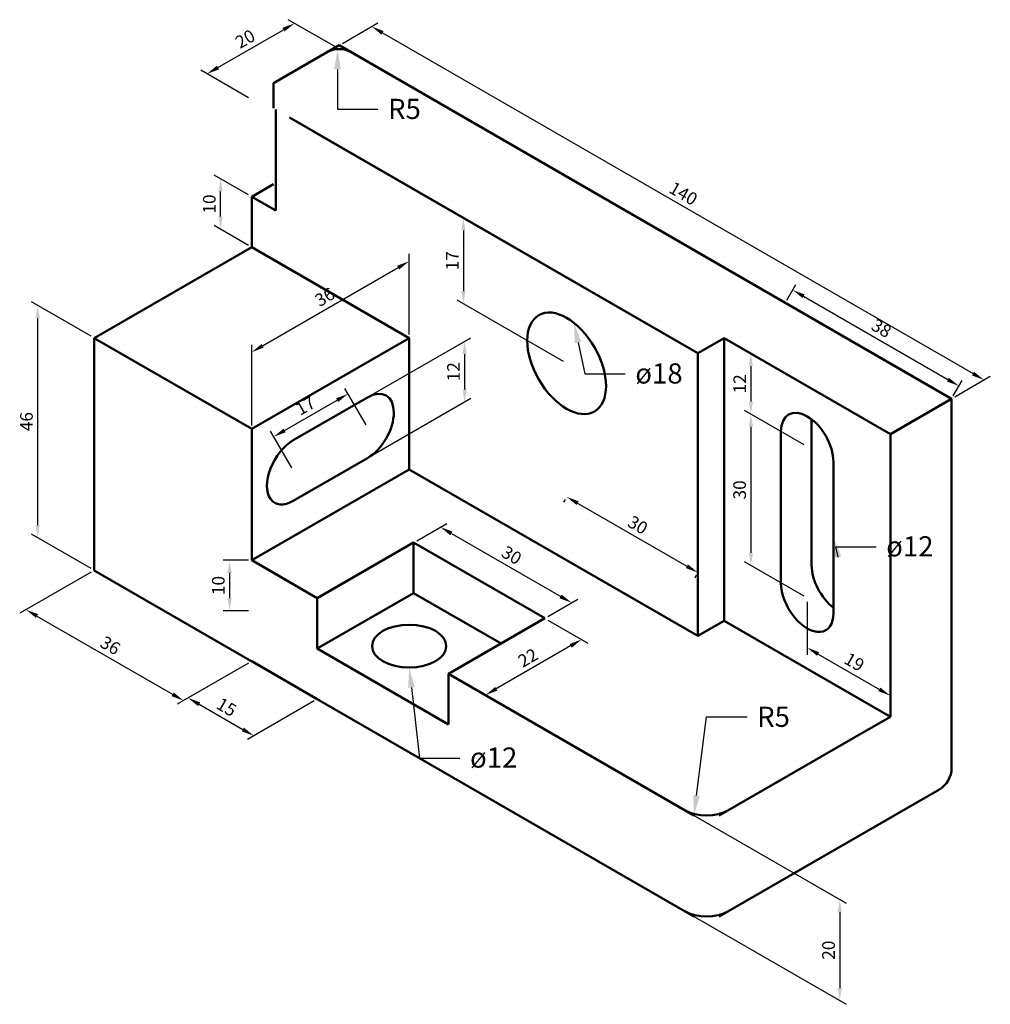
# Model space of a CAD drawing. Units: millimetres. Extents: x 2409 to 2602, y 2299 to 2494.
import ezdxf
from ezdxf import colors
from ezdxf.entities.mleader import LeaderData, LeaderLine
from ezdxf.math import Vec2, Vec3

# ---------------------------------------------------------------- set-up
doc = ezdxf.new("R2010")
doc.units = ezdxf.units.MM
for name, color, linetype, lineweight in [('M-DIMS', 2, 'Continuous', 25), ('M-OUTL', 7, 'Continuous', 50), ('M-TEXT', 3, 'Continuous', 25)]:
    doc.layers.add(name, color=color, linetype=linetype, lineweight=lineweight)
doc.styles.get("Standard").update_dxf_attribs({"font": 'arial.ttf'})
doc.dimstyles.new('ISO-25', dxfattribs={"dimtxt": 2.5, "dimasz": 2.5, "dimexe": 1.25, "dimexo": 0.625, "dimtad": 1, "dimtxsty": 'Standard', "dimcen": 2.5, "dimadec": 0, "dimazin": 0, "dimtfac": 1, "dimtmove": 0, "dimatfit": 3, "dimfxl": 1, "dimarcsym": 0})

# ---------------------------------------------------------------- blocks, each defined once
blk = doc.blocks.new('*D1')
at = {"layer": 'Defpoints', "color": 0, "transparency": 16777216}
for p in [(2486.5, 2446.55), (2486.5, 2431.33), (2455.32, 2413.33)]:
    blk.add_point(p, dxfattribs=at)
at = {"layer": 'M-DIMS', "color": 0, "lineweight": -2, "transparency": 16777216}
for p, q in [((2486.5, 2432.05), (2486.5, 2447.99)), ((2457.49, 2429.8), (2484.33, 2445.3)), ((2455.32, 2414.05), (2455.32, 2429.99))]:
    blk.add_line(p, q, dxfattribs=at)
at = {"layer": 'M-DIMS', "color": 0, "transparency": 16777216}
for points in [[(2484.12, 2445.66), (2484.54, 2444.94), (2486.5, 2446.55)], [(2457.28, 2430.16), (2457.69, 2429.44), (2455.32, 2428.55)]]:
    blk.add_solid(points, dxfattribs=at)
at = {"layer": 'M-DIMS', "color": 0, "transparency": 16777216, "insert": (2469.96, 2439.2), "char_height": 2.5, "attachment_point": 5, "rotation": 30}
blk.add_mtext('36', dxfattribs=at)
blk = doc.blocks.new('*D2')
at = {"layer": 'Defpoints', "color": 0, "transparency": 16777216}
for p in [(2412.96, 2437.79), (2424.14, 2431.33), (2424.14, 2385.33)]:
    blk.add_point(p, dxfattribs=at)
at = {"layer": 'M-DIMS', "color": 0, "lineweight": -2, "transparency": 16777216}
for p, q in [((2423.52, 2431.69), (2411.71, 2438.51)), ((2412.96, 2394.29), (2412.96, 2435.29)), ((2423.52, 2385.69), (2411.71, 2392.51))]:
    blk.add_line(p, q, dxfattribs=at)
at = {"layer": 'M-DIMS', "color": 0, "transparency": 16777216}
for points in [[(2412.54, 2435.29), (2413.37, 2435.29), (2412.96, 2437.79)], [(2412.54, 2394.29), (2413.37, 2394.29), (2412.96, 2391.79)]]:
    blk.add_solid(points, dxfattribs=at)
at = {"layer": 'M-DIMS', "color": 0, "transparency": 16777216, "insert": (2411.05, 2414.79), "char_height": 2.5, "attachment_point": 5, "rotation": 90}
blk.add_mtext('46', dxfattribs=at)
blk = doc.blocks.new('*D3')
at = {"layer": 'Defpoints', "color": 0, "transparency": 16777216}
for p in [(2424.14, 2385.33), (2455.32, 2367.33), (2441.82, 2359.54)]:
    blk.add_point(p, dxfattribs=at)
at = {"layer": 'M-DIMS', "color": 0, "lineweight": -2, "transparency": 16777216}
for p, q in [((2423.52, 2384.97), (2409.39, 2376.82)), ((2412.81, 2376.29), (2439.65, 2360.79)), ((2454.7, 2366.97), (2440.57, 2358.82))]:
    blk.add_line(p, q, dxfattribs=at)
at = {"layer": 'M-DIMS', "color": 0, "transparency": 16777216}
for points in [[(2413.02, 2376.65), (2412.6, 2375.93), (2410.64, 2377.54)], [(2439.86, 2361.15), (2439.45, 2360.43), (2441.82, 2359.54)]]:
    blk.add_solid(points, dxfattribs=at)
at = {"layer": 'M-DIMS', "color": 0, "transparency": 16777216, "insert": (2427.18, 2370.18), "char_height": 2.5, "attachment_point": 5, "rotation": 330}
blk.add_mtext('36', dxfattribs=at)
blk = doc.blocks.new('*D4')
at = {"layer": 'Defpoints', "color": 0, "transparency": 16777216}
for p in [(2455.32, 2367.33), (2468.31, 2359.83), (2455.73, 2352.57)]:
    blk.add_point(p, dxfattribs=at)
at = {"layer": 'M-DIMS', "color": 0, "lineweight": -2, "transparency": 16777216}
for p, q in [((2454.7, 2366.97), (2441.49, 2359.35)), ((2467.69, 2359.47), (2454.48, 2351.85)), ((2444.91, 2358.82), (2453.57, 2353.82))]:
    blk.add_line(p, q, dxfattribs=at)
at = {"layer": 'M-DIMS', "color": 0, "transparency": 16777216}
for points in [[(2445.12, 2359.18), (2444.7, 2358.46), (2442.74, 2360.07)], [(2453.78, 2354.18), (2453.36, 2353.46), (2455.73, 2352.57)]]:
    blk.add_solid(points, dxfattribs=at)
at = {"layer": 'M-DIMS', "color": 0, "transparency": 16777216, "insert": (2450.19, 2357.97), "char_height": 2.5, "attachment_point": 5, "rotation": 330}
blk.add_mtext('15', dxfattribs=at)
blk = doc.blocks.new('*D5')
at = {"layer": 'Defpoints', "color": 0, "transparency": 16777216}
for p in [(2455.32, 2387.33), (2450.95, 2377.33), (2455.32, 2377.33)]:
    blk.add_point(p, dxfattribs=at)
at = {"layer": 'M-DIMS', "color": 0, "lineweight": -2, "transparency": 16777216}
for p, q in [((2454.7, 2387.33), (2449.7, 2387.33)), ((2450.95, 2384.83), (2450.95, 2379.83)), ((2454.7, 2377.33), (2449.7, 2377.33))]:
    blk.add_line(p, q, dxfattribs=at)
at = {"layer": 'M-DIMS', "color": 0, "transparency": 16777216}
for points in [[(2450.53, 2384.83), (2451.36, 2384.83), (2450.95, 2387.33)], [(2450.53, 2379.83), (2451.36, 2379.83), (2450.95, 2377.33)]]:
    blk.add_solid(points, dxfattribs=at)
at = {"layer": 'M-DIMS', "color": 0, "transparency": 16777216, "insert": (2449.04, 2382.33), "char_height": 2.5, "attachment_point": 5, "rotation": 90}
blk.add_mtext('10', dxfattribs=at)
blk = doc.blocks.new('*D6')
at = {"layer": 'Defpoints', "color": 0, "transparency": 16777216}
for p in [(2487.36, 2390.83), (2518.67, 2378.91), (2513.34, 2375.83)]:
    blk.add_point(p, dxfattribs=at)
at = {"layer": 'M-DIMS', "color": 0, "lineweight": -2, "transparency": 16777216}
for p, q in [((2487.99, 2391.19), (2493.94, 2394.63)), ((2494.85, 2392.66), (2516.5, 2380.16)), ((2513.97, 2376.19), (2519.92, 2379.63))]:
    blk.add_line(p, q, dxfattribs=at)
at = {"layer": 'M-DIMS', "color": 0, "transparency": 16777216}
for points in [[(2495.06, 2393.02), (2494.64, 2392.29), (2492.69, 2393.91)], [(2516.71, 2380.52), (2516.29, 2379.79), (2518.67, 2378.91)]]:
    blk.add_solid(points, dxfattribs=at)
at = {"layer": 'M-DIMS', "color": 0, "transparency": 16777216, "insert": (2506.63, 2388.05), "char_height": 2.5, "attachment_point": 5, "rotation": 330}
blk.add_mtext('30', dxfattribs=at)
blk = doc.blocks.new('*D7')
at = {"layer": 'Defpoints', "color": 0, "transparency": 16777216}
for p in [(2513.34, 2375.83), (2494.29, 2364.83), (2501.58, 2360.62)]:
    blk.add_point(p, dxfattribs=at)
at = {"layer": 'M-DIMS', "color": 0, "lineweight": -2, "transparency": 16777216}
for p, q in [((2513.97, 2375.47), (2521.88, 2370.9)), ((2518.47, 2370.37), (2503.75, 2361.87)), ((2494.92, 2364.47), (2502.83, 2359.9))]:
    blk.add_line(p, q, dxfattribs=at)
at = {"layer": 'M-DIMS', "color": 0, "transparency": 16777216}
for points in [[(2518.26, 2370.74), (2518.68, 2370.01), (2520.63, 2371.62)], [(2503.54, 2362.24), (2503.95, 2361.51), (2501.58, 2360.62)]]:
    blk.add_solid(points, dxfattribs=at)
at = {"layer": 'M-DIMS', "color": 0, "transparency": 16777216, "insert": (2510.17, 2367.75), "char_height": 2.5, "attachment_point": 5, "rotation": 30}
blk.add_mtext('22', dxfattribs=at)
blk = doc.blocks.new('*D8')
at = {"layer": 'Defpoints', "color": 0, "transparency": 16777216}
for p in [(2449.16, 2462.89), (2455.32, 2459.33), (2455.32, 2449.33)]:
    blk.add_point(p, dxfattribs=at)
at = {"layer": 'M-DIMS', "color": 0, "lineweight": -2, "transparency": 16777216}
for p, q in [((2454.7, 2459.69), (2447.91, 2463.61)), ((2449.16, 2455.39), (2449.16, 2460.39)), ((2454.7, 2449.69), (2447.91, 2453.61))]:
    blk.add_line(p, q, dxfattribs=at)
at = {"layer": 'M-DIMS', "color": 0, "transparency": 16777216}
for points in [[(2448.75, 2460.39), (2449.58, 2460.39), (2449.16, 2462.89)], [(2448.75, 2455.39), (2449.58, 2455.39), (2449.16, 2452.89)]]:
    blk.add_solid(points, dxfattribs=at)
at = {"layer": 'M-DIMS', "color": 0, "transparency": 16777216, "insert": (2447.26, 2457.89), "char_height": 2.5, "attachment_point": 5, "rotation": 90}
blk.add_mtext('10', dxfattribs=at)
blk = doc.blocks.new('*D9')
at = {"layer": 'Defpoints', "color": 0, "transparency": 16777216}
for p in [(2463.8, 2493.66), (2472.64, 2488.56), (2455.32, 2478.56)]:
    blk.add_point(p, dxfattribs=at)
at = {"layer": 'M-DIMS', "color": 0, "lineweight": -2, "transparency": 16777216}
for p, q in [((2472.02, 2488.92), (2462.55, 2494.39)), ((2448.64, 2484.91), (2461.63, 2492.41)), ((2454.7, 2478.92), (2445.23, 2484.39))]:
    blk.add_line(p, q, dxfattribs=at)
at = {"layer": 'M-DIMS', "color": 0, "transparency": 16777216}
for points in [[(2461.42, 2492.78), (2461.84, 2492.05), (2463.8, 2493.66)], [(2448.43, 2485.28), (2448.85, 2484.55), (2446.48, 2483.66)]]:
    blk.add_solid(points, dxfattribs=at)
at = {"layer": 'M-DIMS', "color": 0, "transparency": 16777216, "insert": (2454.19, 2490.31), "char_height": 2.5, "attachment_point": 5, "rotation": 30}
blk.add_mtext('20', dxfattribs=at)
blk = doc.blocks.new('*D10')
at = {"layer": 'Defpoints', "color": 0, "transparency": 16777216}
for p in [(2474.4, 2420.29), (2478.27, 2413.58), (2463.55, 2405.08)]:
    blk.add_point(p, dxfattribs=at)
at = {"layer": 'M-DIMS', "color": 0, "lineweight": -2, "transparency": 16777216}
for p, q in [((2477.96, 2414.12), (2473.78, 2421.37)), ((2461.84, 2413.04), (2472.24, 2419.04)), ((2463.24, 2405.62), (2459.05, 2412.87))]:
    blk.add_line(p, q, dxfattribs=at)
at = {"layer": 'M-DIMS', "color": 0, "transparency": 16777216}
for points in [[(2472.03, 2419.4), (2472.44, 2418.67), (2474.4, 2420.29)], [(2461.64, 2413.4), (2462.05, 2412.67), (2459.68, 2411.79)]]:
    blk.add_solid(points, dxfattribs=at)
at = {"layer": 'M-DIMS', "color": 0, "transparency": 16777216, "insert": (2466.1, 2417.66), "char_height": 2.5, "attachment_point": 5, "rotation": 30}
blk.add_mtext('17', dxfattribs=at)
blk = doc.blocks.new('*D11')
at = {"layer": 'Defpoints', "color": 0, "transparency": 16777216}
for p in [(2476.54, 2418.58), (2497.48, 2418.67), (2476.54, 2406.58)]:
    blk.add_point(p, dxfattribs=at)
at = {"layer": 'M-DIMS', "color": 0, "lineweight": -2, "transparency": 16777216}
for p, q in [((2477.16, 2418.94), (2498.73, 2431.4)), ((2497.48, 2428.17), (2497.48, 2421.17)), ((2477.16, 2406.94), (2498.73, 2419.4))]:
    blk.add_line(p, q, dxfattribs=at)
at = {"layer": 'M-DIMS', "color": 0, "transparency": 16777216}
for points in [[(2497.06, 2428.17), (2497.9, 2428.17), (2497.48, 2430.67)], [(2497.06, 2421.17), (2497.9, 2421.17), (2497.48, 2418.67)]]:
    blk.add_solid(points, dxfattribs=at)
at = {"layer": 'M-DIMS', "color": 0, "transparency": 16777216, "insert": (2495.6, 2424.67), "char_height": 2.5, "attachment_point": 5, "rotation": 90}
blk.add_mtext('12', dxfattribs=at)
blk = doc.blocks.new('*D12')
at = {"layer": 'Defpoints', "color": 0, "transparency": 16777216}
for p in [(2517.68, 2443.33), (2497.23, 2438.14), (2517.68, 2426.33)]:
    blk.add_point(p, dxfattribs=at)
at = {"layer": 'M-DIMS', "color": 0, "lineweight": -2, "transparency": 16777216}
for p, q in [((2517.05, 2443.69), (2495.98, 2455.86)), ((2497.23, 2452.64), (2497.23, 2440.64)), ((2517.05, 2426.69), (2495.98, 2438.86))]:
    blk.add_line(p, q, dxfattribs=at)
at = {"layer": 'M-DIMS', "color": 0, "transparency": 16777216}
for points in [[(2496.82, 2452.64), (2497.65, 2452.64), (2497.23, 2455.14)], [(2496.82, 2440.64), (2497.65, 2440.64), (2497.23, 2438.14)]]:
    blk.add_solid(points, dxfattribs=at)
at = {"layer": 'M-DIMS', "color": 0, "transparency": 16777216, "insert": (2495.35, 2446.64), "char_height": 2.5, "attachment_point": 5, "rotation": 90}
blk.add_mtext('17', dxfattribs=at)
blk = doc.blocks.new('*D13')
at = {"layer": 'Defpoints', "color": 0, "transparency": 16777216}
for p in [(2517.68, 2399.89), (2543.66, 2384.89), (2543.66, 2384.89)]:
    blk.add_point(p, dxfattribs=at)
at = {"layer": 'M-DIMS', "color": 0, "lineweight": -2, "transparency": 16777216}
for p, q in [((2517.36, 2399.35), (2517.05, 2398.81)), ((2519.84, 2398.64), (2541.49, 2386.14)), ((2543.34, 2384.35), (2543.03, 2383.81))]:
    blk.add_line(p, q, dxfattribs=at)
at = {"layer": 'M-DIMS', "color": 0, "transparency": 16777216}
for points in [[(2520.05, 2399), (2519.63, 2398.28), (2517.68, 2399.89)], [(2541.7, 2386.5), (2541.28, 2385.78), (2543.66, 2384.89)]]:
    blk.add_solid(points, dxfattribs=at)
at = {"layer": 'M-DIMS', "color": 0, "transparency": 16777216, "insert": (2531.62, 2394.04), "char_height": 2.5, "attachment_point": 5, "rotation": 330}
blk.add_mtext('30', dxfattribs=at)
blk = doc.blocks.new('*D14')
at = {"layer": 'Defpoints', "color": 0, "transparency": 16777216}
for p in [(2565.31, 2409.83), (2554.15, 2386.27), (2565.31, 2379.83)]:
    blk.add_point(p, dxfattribs=at)
at = {"layer": 'M-DIMS', "color": 0, "lineweight": -2, "transparency": 16777216}
for p, q in [((2564.68, 2410.19), (2552.9, 2417)), ((2554.15, 2413.77), (2554.15, 2388.77)), ((2564.68, 2380.19), (2552.9, 2387))]:
    blk.add_line(p, q, dxfattribs=at)
at = {"layer": 'M-DIMS', "color": 0, "transparency": 16777216}
for points in [[(2553.73, 2413.77), (2554.57, 2413.77), (2554.15, 2416.27)], [(2553.73, 2388.77), (2554.57, 2388.77), (2554.15, 2386.27)]]:
    blk.add_solid(points, dxfattribs=at)
at = {"layer": 'M-DIMS', "color": 0, "transparency": 16777216, "insert": (2552.25, 2401.27), "char_height": 2.5, "attachment_point": 5, "rotation": 90}
blk.add_mtext('30', dxfattribs=at)
blk = doc.blocks.new('*D15')
at = {"layer": 'Defpoints', "color": 0, "transparency": 16777216}
for p in [(2565.31, 2421.83), (2554.15, 2416.27), (2565.31, 2409.83)]:
    blk.add_point(p, dxfattribs=at)
at = {"layer": 'M-DIMS', "color": 0, "lineweight": -2, "transparency": 16777216}
for p, q in [((2564.68, 2422.19), (2552.9, 2429)), ((2554.15, 2425.77), (2554.15, 2418.77)), ((2564.68, 2410.19), (2552.9, 2417))]:
    blk.add_line(p, q, dxfattribs=at)
at = {"layer": 'M-DIMS', "color": 0, "transparency": 16777216}
for points in [[(2553.73, 2425.77), (2554.57, 2425.77), (2554.15, 2428.27)], [(2553.73, 2418.77), (2554.57, 2418.77), (2554.15, 2416.27)]]:
    blk.add_solid(points, dxfattribs=at)
at = {"layer": 'M-DIMS', "color": 0, "transparency": 16777216, "insert": (2552.27, 2422.27), "char_height": 2.5, "attachment_point": 5, "rotation": 90}
blk.add_mtext('12', dxfattribs=at)
blk = doc.blocks.new('*D16')
at = {"layer": 'Defpoints', "color": 0, "transparency": 16777216}
for p in [(2565.31, 2379.83), (2581.76, 2370.33), (2581.76, 2360.51)]:
    blk.add_point(p, dxfattribs=at)
at = {"layer": 'M-DIMS', "color": 0, "lineweight": -2, "transparency": 16777216}
for p, q in [((2565.31, 2379.11), (2565.31, 2368.57)), ((2581.76, 2369.61), (2581.76, 2359.07)), ((2567.47, 2368.76), (2579.6, 2361.76))]:
    blk.add_line(p, q, dxfattribs=at)
at = {"layer": 'M-DIMS', "color": 0, "transparency": 16777216}
for points in [[(2567.68, 2369.12), (2567.26, 2368.4), (2565.31, 2370.01)], [(2579.8, 2362.12), (2579.39, 2361.4), (2581.76, 2360.51)]]:
    blk.add_solid(points, dxfattribs=at)
at = {"layer": 'M-DIMS', "color": 0, "transparency": 16777216, "insert": (2574.48, 2366.91), "char_height": 2.5, "attachment_point": 5, "rotation": 330}
blk.add_mtext('19', dxfattribs=at)
blk = doc.blocks.new('*D17')
at = {"layer": 'Defpoints', "color": 0, "transparency": 16777216}
for p in [(2472.64, 2489.33), (2600.3, 2423.04), (2593.89, 2419.33)]:
    blk.add_point(p, dxfattribs=at)
at = {"layer": 'M-DIMS', "color": 0, "lineweight": -2, "transparency": 16777216}
for p, q in [((2473.27, 2489.69), (2480.31, 2493.76)), ((2481.22, 2491.79), (2598.14, 2424.29)), ((2594.51, 2419.69), (2601.55, 2423.76))]:
    blk.add_line(p, q, dxfattribs=at)
at = {"layer": 'M-DIMS', "color": 0, "transparency": 16777216}
for points in [[(2481.43, 2492.15), (2481.02, 2491.43), (2479.06, 2493.04)], [(2598.35, 2424.65), (2597.93, 2423.93), (2600.3, 2423.04)]]:
    blk.add_solid(points, dxfattribs=at)
at = {"layer": 'M-DIMS', "color": 0, "transparency": 16777216, "insert": (2540.63, 2459.68), "char_height": 2.5, "attachment_point": 5, "rotation": 330}
blk.add_mtext('140', dxfattribs=at)
blk = doc.blocks.new('*D18')
at = {"layer": 'Defpoints', "color": 0, "transparency": 16777216}
for p in [(2560.98, 2438.33), (2595.34, 2421.85), (2593.89, 2419.33)]:
    blk.add_point(p, dxfattribs=at)
at = {"layer": 'M-DIMS', "color": 0, "lineweight": -2, "transparency": 16777216}
for p, q in [((2561.29, 2438.87), (2563.05, 2441.93)), ((2564.59, 2439.6), (2593.17, 2423.1)), ((2594.2, 2419.87), (2595.96, 2422.93))]:
    blk.add_line(p, q, dxfattribs=at)
at = {"layer": 'M-DIMS', "color": 0, "transparency": 16777216}
for points in [[(2564.8, 2439.96), (2564.39, 2439.24), (2562.43, 2440.85)], [(2593.38, 2423.46), (2592.97, 2422.74), (2595.34, 2421.85)]]:
    blk.add_solid(points, dxfattribs=at)
at = {"layer": 'M-DIMS', "color": 0, "transparency": 16777216, "insert": (2579.84, 2433), "char_height": 2.5, "attachment_point": 5, "rotation": 330}
blk.add_mtext('38', dxfattribs=at)
blk = doc.blocks.new('*D19')
at = {"layer": 'Defpoints', "color": 0, "transparency": 16777216}
for p in [(2538.57, 2339.27), (2538.57, 2319.27), (2571.75, 2300.11)]:
    blk.add_point(p, dxfattribs=at)
at = {"layer": 'M-DIMS', "color": 0, "lineweight": -2, "transparency": 16777216}
for p, q in [((2539.2, 2338.91), (2573, 2319.39)), ((2539.2, 2318.91), (2573, 2299.39)), ((2571.75, 2317.61), (2571.75, 2302.61))]:
    blk.add_line(p, q, dxfattribs=at)
at = {"layer": 'M-DIMS', "color": 0, "transparency": 16777216}
for points in [[(2571.33, 2317.61), (2572.17, 2317.61), (2571.75, 2320.11)], [(2571.33, 2302.61), (2572.17, 2302.61), (2571.75, 2300.11)]]:
    blk.add_solid(points, dxfattribs=at)
at = {"layer": 'M-DIMS', "color": 0, "transparency": 16777216, "insert": (2569.85, 2310.11), "char_height": 2.5, "attachment_point": 5, "rotation": 90}
blk.add_mtext('20', dxfattribs=at)

msp = doc.modelspace()

# ---------------------------------------------------------------- linework, layer by layer
at = {"layer": 'M-OUTL'}
for p, q in [((2459.651, 2481.832), (2472.642, 2489.332)), ((2593.885, 2419.332), (2472.642, 2489.332)), ((2470.142, 2487.889), (2462.821, 2483.663)), ((2475.142, 2487.889), (2593.885, 2419.332)), ((2459.651, 2476.832), (2459.651, 2481.832)), ((2460.084, 2456.582), (2460.084, 2476.582)), ((2543.656, 2428.332), (2462.821, 2475.002)), ((2467.584, 2472.252), (2543.656, 2428.332)), ((2459.651, 2461.832), (2455.321, 2459.332)), ((2455.321, 2449.332), (2455.321, 2459.332)), ((2455.321, 2459.332), (2460.084, 2456.582)), ((2455.321, 2449.332), (2424.144, 2431.332)), ((2455.321, 2449.332), (2486.498, 2431.332)), ((2586.385, 2423.663), (2560.976, 2438.332)), ((2424.144, 2431.332), (2424.144, 2385.332)), ((2455.321, 2413.332), (2424.144, 2431.332)), ((2486.498, 2431.332), (2455.321, 2413.332)), ((2486.498, 2431.332), (2486.498, 2405.332)), ((2543.656, 2428.332), (2548.852, 2431.332)), ((2581.761, 2412.332), (2548.852, 2431.332)), ((2548.852, 2431.332), (2548.852, 2375.332)), ((2543.656, 2428.332), (2543.656, 2372.332)), ((2463.548, 2411.082), (2478.271, 2419.582)), ((2581.761, 2412.332), (2593.885, 2419.332)), ((2593.885, 2419.332), (2593.885, 2346.219)), ((2566.172, 2415.248), (2566.172, 2386.332)), ((2586.385, 2415.002), (2581.761, 2412.332)), ((2455.321, 2403.332), (2455.321, 2413.332)), ((2455.321, 2413.332), (2455.321, 2387.332)), ((2560.11, 2412.832), (2560.11, 2382.832)), ((2581.761, 2412.332), (2581.761, 2356.332)), ((2463.548, 2399.082), (2478.271, 2407.582)), ((2570.503, 2406.832), (2570.503, 2376.832)), ((2486.498, 2405.332), (2455.321, 2387.332)), ((2543.656, 2372.332), (2486.498, 2405.332)), ((2487.364, 2390.832), (2468.312, 2379.832)), ((2513.345, 2375.832), (2487.364, 2390.832)), ((2487.364, 2380.832), (2487.364, 2390.832)), ((2468.312, 2379.832), (2455.321, 2387.332)), ((2542.888, 2316.776), (2424.144, 2385.332)), ((2468.312, 2369.832), (2487.364, 2380.832)), ((2468.312, 2369.832), (2468.312, 2379.832)), ((2468.312, 2379.832), (2468.312, 2369.832)), ((2487.364, 2380.832), (2504.685, 2370.832)), ((2494.292, 2364.832), (2513.345, 2375.832)), ((2543.656, 2372.332), (2548.852, 2375.332)), ((2548.852, 2375.332), (2581.761, 2356.332)), ((2468.312, 2369.832), (2494.292, 2354.832)), ((2455.321, 2367.332), (2468.312, 2359.832)), ((2542.888, 2336.776), (2494.292, 2364.832)), ((2494.292, 2354.832), (2494.292, 2364.832)), ((2576.565, 2353.332), (2581.761, 2356.332)), ((2547.888, 2336.776), (2576.565, 2353.332)), ((2591.385, 2341.889), (2562.708, 2325.332)), ((2576.565, 2333.332), (2547.888, 2316.776))]:
    msp.add_line(p, q, dxfattribs=at)
for centre, start, end in [((2472.642, 2483.559), 60, 120), ((2588.885, 2346.219), 300, 0)]:
    msp.add_arc(centre, 5, start, end, dxfattribs=at)
for centre, major_axis in [((2517.675, 2426.332), (5.511, -9.546)), ((2486.498, 2370.332), (-7.348, 0))]:
    msp.add_ellipse(centre, major_axis=major_axis, ratio=0.5773503, dxfattribs=at)
for centre, major_axis, start_param, end_param in [((2478.271, 2413.582), (-3.674, -6.364), 7.0685835, 10.2101761), ((2565.306, 2409.832), (3.674, -6.364), 7.0685835, 10.2101761), ((2463.548, 2405.082), (-3.674, -6.364), 3.9269908, 7.0685835), ((2571.369, 2383.332), (3.674, -6.364), 3.9269908, 5.3303391), ((2565.306, 2379.832), (3.674, -6.364), 3.9269908, 7.0685835), ((2545.388, 2340.332), (6.124, 0), 3.9269908, 5.4977871), ((2545.388, 2320.332), (6.124, 0), 3.9269908, 5.4977871)]:
    msp.add_ellipse(centre, major_axis=major_axis, ratio=0.5773503, start_param=start_param, end_param=end_param, dxfattribs=at)

# ---------------------------------------------------------------- dimensions: what is measured, and where the dimension line sits
at = {"layer": 'M-DIMS'}
for p1, p2, distance, picture, middle in [((2455.321, 2478.559), (2472.642, 2488.559), 8.844, '*D9', (2454.187, 2490.312)), ((2472.642, 2489.332), (2593.885, 2419.332), 6.417, '*D17', (2540.631, 2459.684)), ((2455.321, 2449.332), (2455.321, 2459.332), 6.157, '*D8', (2447.263, 2457.887)), ((2517.675, 2443.332), (2517.675, 2426.332), -20.443, '*D12', (2495.352, 2446.635)), ((2455.321, 2413.332), (2486.498, 2431.332), 13.179, '*D1', (2469.959, 2439.198)), ((2560.976, 2438.332), (2593.885, 2419.332), 2.907, '*D18', (2579.835, 2432.997)), ((2424.144, 2385.332), (2424.144, 2431.332), 11.189, '*D2', (2411.054, 2414.793)), ((2476.538, 2418.582), (2476.538, 2406.582), 20.944, '*D11', (2495.601, 2424.674)), ((2565.306, 2421.832), (2565.306, 2409.832), -11.158, '*D15', (2552.268, 2422.274)), ((2463.548, 2405.082), (2478.271, 2413.582), 7.74, '*D10', (2466.1, 2417.663)), ((2565.306, 2409.832), (2565.306, 2379.832), -11.158, '*D14', (2552.246, 2401.274)), ((2517.675, 2399.893), (2543.656, 2384.893), 0, '*D13', (2531.617, 2394.04)), ((2487.364, 2390.832), (2513.345, 2375.832), 5.322, '*D6', (2506.628, 2388.053)), ((2455.321, 2387.332), (2455.321, 2377.332), -4.376, '*D5', (2449.044, 2382.332)), ((2424.144, 2385.332), (2455.321, 2367.332), -13.501, '*D3', (2427.183, 2370.185)), ((2565.306, 2379.832), (2581.761, 2370.332), -8.504, '*D16', (2574.484, 2366.909)), ((2513.345, 2375.832), (2494.292, 2364.832), 7.288, '*D7', (2510.167, 2367.753)), ((2455.321, 2367.332), (2468.312, 2359.832), -12.58, '*D4', (2450.188, 2357.966)), ((2538.571, 2339.268), (2538.571, 2319.268), 33.179, '*D19', (2569.849, 2310.112))]:
    dim = msp.add_aligned_dim(p1=p1, p2=p2, distance=distance, dimstyle='ISO-25', override={"dimclrd": 0, "dimclre": 0, "dimclrt": 0}, dxfattribs=at)
    dim.commit()
    dim.dimension.update_dxf_attribs({"geometry": picture, "text_midpoint": middle})

# ---------------------------------------------------------------- leaders
at = {"layer": 'M-TEXT'}
ml = msp.add_multileader_mtext('Standard', dxfattribs=at)
ml.set_content('R5', color=256)
ml.set_leader_properties()
ml.build(insert=Vec2(0, 0))
ctx = ml.context
ctx.base_point, ctx.plane_origin = Vec3(2480.321, 2476.686), Vec3(2472.321, 2488.549)
notes = []
notes.append((ctx, [(0, (1, 1, 0), (2472.321, 2476.686), (1, 0), 8, [(0, [(2472.321, 2488.549)], 0, [])])]))
ctx.mtext.insert, ctx.mtext.flow_direction = Vec3(2482.321, 2478.72), 5
ml = msp.add_multileader_mtext('Standard', dxfattribs=at)
ml.set_content('ø18', color=256)
ml.set_leader_properties()
ml.build(insert=Vec2(0, 0))
ctx = ml.context
ctx.base_point, ctx.plane_origin = Vec3(2529.277, 2424.224), Vec3(2519.103, 2434.356)
notes.append((ctx, [(0, (1, 1, 0), (2521.277, 2424.224), (1, 0), 8, [(0, [(2519.103, 2434.356)], 0, [])])]))
ctx.mtext.insert, ctx.mtext.flow_direction = Vec3(2531.277, 2426.332), 5
ml = msp.add_multileader_mtext('Standard', dxfattribs=at)
ml.set_content('ø12', color=256)
ml.set_leader_properties()
ml.build(insert=Vec2(0, 0))
ctx = ml.context
ctx.base_point, ctx.plane_origin = Vec3(2578.946, 2389.981), Vec3(2570.503, 2391.832)
notes.append((ctx, [(0, (1, 1, 0), (2570.946, 2389.981), (1, 0), 8, [(0, [(2570.503, 2391.832)], 0, [])])]))
ctx.mtext.insert, ctx.mtext.flow_direction = Vec3(2580.946, 2392.088), 5
ml = msp.add_multileader_mtext('Standard', dxfattribs=at)
ml.set_content('ø12', color=256)
ml.set_leader_properties()
ml.build(insert=Vec2(0, 0))
ctx = ml.context
ctx.base_point, ctx.plane_origin = Vec3(2496.552, 2348.147), Vec3(2486.498, 2366.09)
notes.append((ctx, [(0, (1, 1, 0), (2488.552, 2348.147), (1, 0), 8, [(0, [(2486.498, 2366.09)], 0, [])])]))
ctx.mtext.insert, ctx.mtext.flow_direction = Vec3(2498.552, 2350.254), 5
ml = msp.add_multileader_mtext('Standard', dxfattribs=at)
ml.set_content('R5', color=256)
ml.set_leader_properties()
ml.build(insert=Vec2(0, 0))
ctx = ml.context
ctx.base_point, ctx.plane_origin = Vec3(2553.388, 2356.3), Vec3(2542.888, 2336.776)
notes.append((ctx, [(0, (1, 1, 0), (2545.388, 2356.3), (1, 0), 8, [(0, [(2542.888, 2336.776)], 0, [])])]))
ctx.mtext.insert, ctx.mtext.flow_direction = Vec3(2555.388, 2358.334), 5
for ctx, leaders in notes:
    for number, flags, end, landing, length, lines in leaders:
        leader = LeaderData()
        leader.index, (leader.has_last_leader_line, leader.has_dogleg_vector, leader.attachment_direction) = number, flags
        leader.last_leader_point, leader.dogleg_vector, leader.dogleg_length = Vec3(end), Vec3(landing), length
        for number, points, colour, breaks in lines:
            line = LeaderLine()
            line.index, line.vertices, line.color, line.breaks = number, Vec3.list(points), colors.encode_raw_color(colour), breaks
            leader.lines.append(line)
        ctx.leaders.append(leader)

doc.saveas('drawing.dxf')
